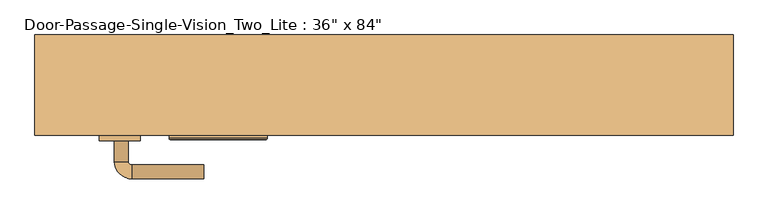
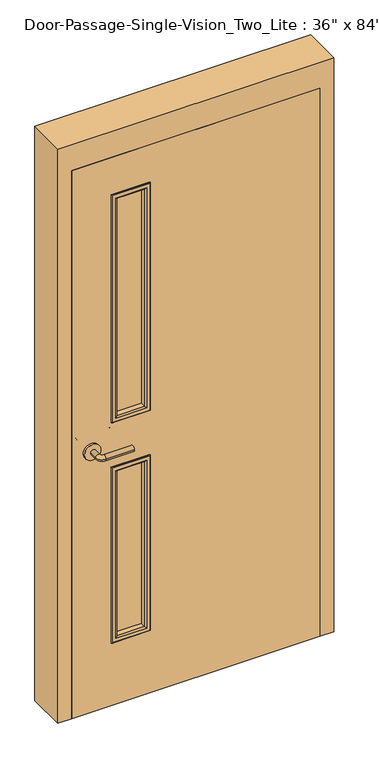
"""IFC4 building model written with IfcOpenShell, lengths in millimetres: door geometry."""

from ifc_helpers import new_model, si_unit, point, frame, frame_2d, origin, place, context, project, spatial, polyline, circle_curve, ellipse_curve, trimmed, segment, composite_curve, outline, extrude, faceted_brep, source, transform, mapped, element, save
from ifc_brep_helpers import plane_surface, cylinder_surface, revolved_surface, advanced_brep


def door_52fb15b9(model_context):
    return source(origin(), model_context, "Body", "SolidModel", [
        advanced_brep(
        [(-392.190625, -68.2, 1016.0), (-372.190625, -68.2, 1016.0), (-392.190625, -38.2, 1016.0), (-372.190625, -38.2, 1016.0), (-367.190625, -33.2, 1016.0), (-367.190625, -13.2, 1016.0), (-262.190625, -13.2, 1016.0), (-262.190625, -33.2, 1016.0)],
        [
            (0, 1, circle_curve(frame((-382.190625, -68.2, 1016.0), z_axis=(0.0, -1.0, 0.0), x_axis=(1.0, 0.0, 0.0)), 10.0)),
            (1, 0, circle_curve(frame((-382.190625, -68.2, 1016.0), z_axis=(0.0, -1.0, 0.0), x_axis=(1.0, 0.0, 0.0)), 10.0)),
            (0, 2),
            (2, 3, circle_curve(frame((-382.190625, -38.2, 1016.0), z_axis=(0.0, -1.0, 0.0), x_axis=(1.0, 0.0, 0.0)), 10.0)),
            (3, 1),
            (3, 2, circle_curve(frame((-382.190625, -38.2, 1016.0), z_axis=(0.0, -1.0, 0.0), x_axis=(1.0, 0.0, 0.0)), 10.0)),
            (4, 3, circle_curve(frame((-367.190625, -38.2, 1016.0), z_axis=(0.0, 0.0, 1.0), x_axis=(-1.0, 0.0, 0.0)), 5.0)),
            (2, 5, circle_curve(frame((-367.190625, -38.2, 1016.0), z_axis=(0.0, 0.0, -1.0), x_axis=(-1.0, 0.0, 0.0)), 25.0)),
            (5, 4, circle_curve(frame((-367.190625, -23.2, 1016.0), z_axis=(-1.0, 0.0, 0.0), x_axis=(0.0, -1.0, 0.0)), 10.0)),
            (4, 5, circle_curve(frame((-367.190625, -23.2, 1016.0), z_axis=(-1.0, 0.0, 0.0), x_axis=(0.0, -1.0, 0.0)), 10.0)),
            (6, 7, circle_curve(frame((-262.190625, -23.2, 1016.0), z_axis=(1.0, 0.0, 0.0), x_axis=(0.0, -1.0, 0.0)), 10.0)),
            (7, 6, circle_curve(frame((-262.190625, -23.2, 1016.0), z_axis=(1.0, 0.0, 0.0), x_axis=(0.0, -1.0, 0.0)), 10.0)),
            (5, 6),
            (7, 4),
        ],
        [
            plane_surface(frame((-382.190625, -68.2, 1016.0), z_axis=(0.0, -1.0, 0.0), x_axis=(0.0, 0.0, 1.0))),
            cylinder_surface(frame((-382.190625, -68.2, 1016.0), z_axis=(0.0, -1.0, 0.0), x_axis=(1.0, 0.0, 0.0)), 10.0),
            revolved_surface(trimmed(ellipse_curve(frame((-382.190625, -38.2, 1016.0), z_axis=(0.0, -1.0, 0.0), x_axis=(1.0, 0.0, 0.0)), 10.0, 10.0), [point((-392.190625, -38.2, 1016.0))], [point((-372.190625, -38.2, 1016.0))], True, "CARTESIAN"), (-367.190625, -38.2, 1016.0), (0.0, 0.0, -1.0)),
            revolved_surface(trimmed(ellipse_curve(frame((-382.190625, -38.2, 1016.0), z_axis=(0.0, -1.0, 0.0), x_axis=(1.0, 0.0, 0.0)), 10.0, 10.0), [point((-372.190625, -38.2, 1016.0))], [point((-392.190625, -38.2, 1016.0))], True, "CARTESIAN"), (-367.190625, -38.2, 1016.0), (0.0, 0.0, -1.0)),
            plane_surface(frame((-262.190625, -23.2, 1016.0), z_axis=(1.0, 0.0, 0.0), x_axis=(0.0, 0.0, 1.0))),
            cylinder_surface(frame((-367.190625, -23.2, 1016.0), z_axis=(-1.0, 0.0, 0.0), x_axis=(0.0, -1.0, 0.0)), 10.0),
        ],
        [
            (0, [[1, 2]]),
            (1, [[-1, 3, 4, 5]]),
            (1, [[-2, -5, 6, -3]]),
            (2, [[7, -4, 8, 9]]),
            (3, [[-8, -6, -7, 10]]),
            (4, [[11, 12]]),
            (5, [[-9, 13, -12, 14]]),
            (5, [[-10, -14, -11, -13]]),
        ],
    ),
        extrude(outline(composite_curve([segment(trimmed(circle_curve(frame_2d((1016.0, -384.690625)), 30.0), [point((1016.0, -414.690625))], [point((1016.0, -354.690625))], False, "CARTESIAN"), True, "CONTINUOUS"), segment(trimmed(circle_curve(frame_2d((1016.0, -384.690625)), 30.0), [point((1016.0, -354.690625))], [point((1016.0, -414.690625))], False, "CARTESIAN"), True, "CONTINUOUS")], self_intersect=False)), frame((0.0, -76.2, 0.0), z_axis=(0.0, 1.0, 0.0), x_axis=(0.0, 0.0, 1.0)), (0.0, 0.0, 1.0), 8.0),
        advanced_brep(
        [(-392.190625, -128.65, 1016.0), (-372.190625, -128.65, 1016.0), (-372.190625, -158.65, 1016.0), (-392.190625, -158.65, 1016.0), (-367.190625, -163.65, 1016.0), (-367.190625, -183.65, 1016.0), (-262.190625, -183.65, 1016.0), (-262.190625, -163.65, 1016.0)],
        [
            (0, 1, circle_curve(frame((-382.190625, -128.65, 1016.0), z_axis=(0.0, 1.0, 0.0), x_axis=(1.0, 0.0, 0.0)), 10.0)),
            (1, 0, circle_curve(frame((-382.190625, -128.65, 1016.0), z_axis=(0.0, 1.0, 0.0), x_axis=(1.0, 0.0, 0.0)), 10.0)),
            (1, 2),
            (2, 3, circle_curve(frame((-382.190625, -158.65, 1016.0), z_axis=(0.0, 1.0, 0.0), x_axis=(1.0, 0.0, 0.0)), 10.0)),
            (3, 0),
            (3, 2, circle_curve(frame((-382.190625, -158.65, 1016.0), z_axis=(0.0, 1.0, 0.0), x_axis=(1.0, 0.0, 0.0)), 10.0)),
            (4, 5, circle_curve(frame((-367.190625, -173.65, 1016.0), z_axis=(-1.0, 0.0, 0.0), x_axis=(0.0, 1.0, 0.0)), 10.0)),
            (5, 3, circle_curve(frame((-367.190625, -158.65, 1016.0), z_axis=(0.0, 0.0, -1.0), x_axis=(-1.0, 0.0, 0.0)), 25.0)),
            (2, 4, circle_curve(frame((-367.190625, -158.65, 1016.0), z_axis=(0.0, 0.0, 1.0), x_axis=(-1.0, 0.0, 0.0)), 5.0)),
            (5, 4, circle_curve(frame((-367.190625, -173.65, 1016.0), z_axis=(-1.0, 0.0, 0.0), x_axis=(0.0, 1.0, 0.0)), 10.0)),
            (6, 7, circle_curve(frame((-262.190625, -173.65, 1016.0), z_axis=(1.0, 0.0, 0.0), x_axis=(0.0, 1.0, 0.0)), 10.0)),
            (7, 6, circle_curve(frame((-262.190625, -173.65, 1016.0), z_axis=(1.0, 0.0, 0.0), x_axis=(0.0, 1.0, 0.0)), 10.0)),
            (4, 7),
            (6, 5),
        ],
        [
            plane_surface(frame((-382.190625, -128.65, 1016.0), z_axis=(0.0, 1.0, 0.0), x_axis=(0.0, 0.0, 1.0))),
            cylinder_surface(frame((-382.190625, -128.65, 1016.0), z_axis=(0.0, 1.0, 0.0), x_axis=(1.0, 0.0, 0.0)), 10.0),
            revolved_surface(trimmed(ellipse_curve(frame((-382.190625, -158.65, 1016.0), z_axis=(0.0, -1.0, 0.0), x_axis=(1.0, 0.0, 0.0)), 10.0, 10.0), [point((-392.190625, -158.65, 1016.0))], [point((-372.190625, -158.65, 1016.0))], True, "CARTESIAN"), (-367.190625, -158.65, 1016.0), (0.0, 0.0, -1.0)),
            revolved_surface(trimmed(ellipse_curve(frame((-382.190625, -158.65, 1016.0), z_axis=(0.0, -1.0, 0.0), x_axis=(1.0, 0.0, 0.0)), 10.0, 10.0), [point((-372.190625, -158.65, 1016.0))], [point((-392.190625, -158.65, 1016.0))], True, "CARTESIAN"), (-367.190625, -158.65, 1016.0), (0.0, 0.0, -1.0)),
            plane_surface(frame((-262.190625, -173.65, 1016.0), z_axis=(1.0, 0.0, 0.0), x_axis=(0.0, 0.0, 1.0))),
            cylinder_surface(frame((-367.190625, -173.65, 1016.0), z_axis=(-1.0, 0.0, 0.0), x_axis=(0.0, 1.0, 0.0)), 10.0),
        ],
        [
            (0, [[1, 2]]),
            (1, [[3, 4, 5, -2]]),
            (1, [[-5, 6, -3, -1]]),
            (2, [[7, 8, -4, 9]]),
            (3, [[10, -9, -6, -8]]),
            (4, [[11, 12]]),
            (5, [[13, -11, 14, -7]]),
            (5, [[-14, -12, -13, -10]]),
        ],
    ),
        extrude(outline(composite_curve([segment(trimmed(circle_curve(frame_2d((1016.0, -384.690625)), 30.0), [point((1016.0, -414.690625))], [point((1016.0, -354.690625))], False, "CARTESIAN"), True, "CONTINUOUS"), segment(trimmed(circle_curve(frame_2d((1016.0, -384.690625)), 30.0), [point((1016.0, -354.690625))], [point((1016.0, -414.690625))], False, "CARTESIAN"), True, "CONTINUOUS")], self_intersect=False)), frame((0.0, -128.65, 0.0), z_axis=(0.0, 1.0, 0.0), x_axis=(0.0, 0.0, 1.0)), (0.0, 0.0, 1.0), 8.0),
        extrude(outline(polyline([(2133.6, -457.2), (0.0, -457.2), (0.0, 457.2), (2133.6, 457.2), (2133.6, -457.2)]), holes=[polyline([(1981.2, -304.8), (1981.2, -177.8), (1111.25, -177.8), (1111.25, -304.8), (1981.2, -304.8)]), polyline([(920.75, -304.8), (920.75, -177.8), (254.0, -177.8), (254.0, -304.8), (920.75, -304.8)])]), frame((0.0, -120.65, 0.0), z_axis=(0.0, 1.0, 0.0), x_axis=(0.0, 0.0, 1.0)), (0.0, 0.0, 1.0), 44.45),
        faceted_brep([(457.2, -71.4375, 0.0), (441.325, -71.4375, 0.0), (441.325, -23.8125, 0.0), (457.2, -23.8125, 0.0), (457.2, 25.4, 0.0), (508.0, 25.4, 0.0), (508.0, -120.65, 0.0), (457.2, -120.65, 0.0), (457.2, -120.65, 2133.6), (457.2, -71.4375, 2133.6), (508.0, -120.65, 2235.2), (-508.0, -120.65, 2235.2), (-508.0, -120.65, 0.0), (-457.2, -120.65, 0.0), (-457.2, -120.65, 2133.6), (508.0, 25.4, 2235.2), (457.2, 25.4, 2133.6), (-457.2, 25.4, 2133.6), (-457.2, 25.4, 0.0), (-508.0, 25.4, 0.0), (-508.0, 25.4, 2235.2), (457.2, -23.8125, 2133.6), (441.325, -23.8125, 2117.725), (-441.325, -23.8125, 2117.725), (-441.325, -23.8125, 0.0), (-457.2, -23.8125, 0.0), (-457.2, -23.8125, 2133.6), (441.325, -71.4375, 2117.725), (-457.2, -71.4375, 2133.6), (-457.2, -71.4375, 0.0), (-441.325, -71.4375, 0.0), (-441.325, -71.4375, 2117.725)], [[[0, 1, 2, 3, 4, 5, 6, 7]], [[7, 8, 9, 0]], [[6, 10, 11, 12, 13, 14, 8, 7]], [[5, 15, 10, 6]], [[4, 16, 17, 18, 19, 20, 15, 5]], [[3, 21, 16, 4]], [[2, 22, 23, 24, 25, 26, 21, 3]], [[1, 27, 22, 2]], [[0, 9, 28, 29, 30, 31, 27, 1]], [[8, 14, 28, 9]], [[16, 21, 26, 17]], [[22, 27, 31, 23]], [[12, 19, 18, 25, 24, 30, 29, 13]], [[13, 29, 28, 14]], [[11, 20, 19, 12]], [[17, 26, 25, 18]], [[23, 31, 30, 24]], [[15, 20, 11, 10]]]),
        extrude(outline(polyline([(-177.8, -95.25), (-177.8, -101.6), (-304.8, -101.6), (-304.8, -95.25), (-177.8, -95.25)])), frame((0.0, 0.0, 1111.25), z_axis=(0.0, 0.0, 1.0), x_axis=(1.0, 0.0, 0.0)), (0.0, 0.0, 1.0), 869.95),
        extrude(outline(polyline([(-177.8, -95.25), (-177.8, -101.6), (-304.8, -101.6), (-304.8, -95.25), (-177.8, -95.25)])), frame((0.0, 0.0, 254.0), z_axis=(0.0, 0.0, 1.0), x_axis=(1.0, 0.0, 0.0)), (0.0, 0.0, 1.0), 666.75),
        advanced_brep(
        [(-304.8, -101.6, 1981.2), (-304.8, -101.6, 1111.25), (-304.8, -120.65, 1111.25), (-304.8, -120.65, 1981.2), (-292.8, -121.65, 1969.2), (-292.8, -121.65, 1123.25), (-292.8, -101.6, 1123.25), (-292.8, -101.6, 1969.2), (-297.8, -126.65, 1974.2), (-297.8, -126.65, 1118.25), (-312.8, -124.65, 1989.2), (-312.8, -124.65, 1103.25), (-310.8, -126.65, 1105.25), (-310.8, -126.65, 1987.2), (-312.8, -120.65, 1989.2), (-312.8, -120.65, 1103.25), (-177.8, -101.6, 1111.25), (-177.8, -120.65, 1111.25), (-189.8, -121.65, 1123.25), (-189.8, -101.6, 1123.25), (-184.8, -126.65, 1118.25), (-169.8, -124.65, 1103.25), (-171.8, -126.65, 1105.25), (-169.8, -120.65, 1103.25), (-177.8, -101.6, 1981.2), (-177.8, -120.65, 1981.2), (-189.8, -121.65, 1969.2), (-189.8, -101.6, 1969.2), (-184.8, -126.65, 1974.2), (-169.8, -124.65, 1989.2), (-171.8, -126.65, 1987.2), (-169.8, -120.65, 1989.2)],
        [
            (0, 1),
            (1, 2),
            (2, 3),
            (3, 0),
            (4, 5),
            (5, 6),
            (6, 7),
            (7, 4),
            (8, 9),
            (9, 5, ellipse_curve(frame((-297.8, -121.65, 1118.25), z_axis=(-0.7071067811865475, 0.0, 0.7071067811865475), x_axis=(0.7071067811865474, 0.0, 0.7071067811865476)), 7.0710678, 5.0)),
            (4, 8, ellipse_curve(frame((-297.8, -121.65, 1974.2), z_axis=(-0.7071067811865475, 0.0, -0.7071067811865475), x_axis=(-0.7071067811865474, 0.0, 0.7071067811865476)), 7.0710678, 5.0)),
            (10, 11),
            (11, 12, ellipse_curve(frame((-310.8, -124.65, 1105.25), z_axis=(-0.7071067811865475, 0.0, 0.7071067811865475), x_axis=(0.7071067811865474, 0.0, 0.7071067811865476)), 2.8284271, 2.0)),
            (12, 13),
            (13, 10, ellipse_curve(frame((-310.8, -124.65, 1987.2), z_axis=(-0.7071067811865475, 0.0, -0.7071067811865475), x_axis=(-0.7071067811865474, 0.0, 0.7071067811865476)), 2.8284271, 2.0)),
            (14, 15),
            (15, 11),
            (10, 14),
            (1, 16),
            (16, 17),
            (17, 2),
            (5, 18),
            (18, 19),
            (19, 6),
            (9, 20),
            (20, 18, ellipse_curve(frame((-184.8, -121.65, 1118.25), z_axis=(-0.7071067811865475, 0.0, -0.7071067811865475), x_axis=(-0.7071067811865476, 0.0, 0.7071067811865474)), 7.0710678, 5.0)),
            (11, 21),
            (21, 22, ellipse_curve(frame((-171.8, -124.65, 1105.25), z_axis=(-0.7071067811865475, 0.0, -0.7071067811865475), x_axis=(-0.7071067811865476, 0.0, 0.7071067811865474)), 2.8284271, 2.0)),
            (22, 12),
            (15, 23),
            (23, 21),
            (16, 24),
            (24, 25),
            (25, 17),
            (18, 26),
            (26, 27),
            (27, 19),
            (20, 28),
            (28, 26, ellipse_curve(frame((-184.8, -121.65, 1974.2), z_axis=(0.7071067811865475, 0.0, -0.7071067811865475), x_axis=(-0.7071067811865474, 0.0, -0.7071067811865476)), 7.0710678, 5.0)),
            (21, 29),
            (29, 30, ellipse_curve(frame((-171.8, -124.65, 1987.2), z_axis=(0.7071067811865475, 0.0, -0.7071067811865475), x_axis=(-0.7071067811865474, 0.0, -0.7071067811865476)), 2.8284271, 2.0)),
            (30, 22),
            (23, 31),
            (31, 29),
            (14, 31),
            (25, 3),
            (24, 0),
            (27, 7),
            (26, 4),
            (28, 8),
            (30, 13),
            (29, 10),
        ],
        [
            plane_surface(frame((-304.8, -120.65, 1981.2), z_axis=(-1.0, 0.0, 0.0), x_axis=(0.0, 0.0, -1.0))),
            plane_surface(frame((-292.8, -101.6, 1969.2), z_axis=(1.0, 0.0, 0.0), x_axis=(0.0, 0.0, -1.0))),
            cylinder_surface(frame((-297.8, -121.65, 1981.2), z_axis=(0.0, 0.0, 1.0), x_axis=(-1.0, 0.0, 0.0)), 5.0),
            cylinder_surface(frame((-310.8, -124.65, 1981.2), z_axis=(0.0, 0.0, 1.0), x_axis=(-1.0, 0.0, 0.0)), 2.0),
            plane_surface(frame((-312.8, -124.65, 1989.2), z_axis=(-1.0, 0.0, 0.0), x_axis=(0.0, 0.0, -1.0))),
            plane_surface(frame((-304.8, -120.65, 1111.25), z_axis=(0.0, 0.0, -1.0), x_axis=(1.0, 0.0, 0.0))),
            plane_surface(frame((-292.8, -101.6, 1123.25), z_axis=(0.0, 0.0, 1.0), x_axis=(1.0, 0.0, 0.0))),
            cylinder_surface(frame((-304.8, -121.65, 1118.25), z_axis=(-1.0, 0.0, 0.0), x_axis=(0.0, 0.0, -1.0)), 5.0),
            cylinder_surface(frame((-304.8, -124.65, 1105.25), z_axis=(-1.0, 0.0, 0.0), x_axis=(0.0, 0.0, -1.0)), 2.0),
            plane_surface(frame((-312.8, -124.65, 1103.25), z_axis=(0.0, 0.0, -1.0), x_axis=(1.0, 0.0, 0.0))),
            plane_surface(frame((-177.8, -120.65, 1111.25), z_axis=(1.0, 0.0, 0.0), x_axis=(0.0, 0.0, 1.0))),
            plane_surface(frame((-189.8, -101.6, 1123.25), z_axis=(-1.0, 0.0, 0.0), x_axis=(0.0, 0.0, 1.0))),
            cylinder_surface(frame((-184.8, -121.65, 1111.25), z_axis=(0.0, 0.0, -1.0), x_axis=(1.0, 0.0, 0.0)), 5.0),
            cylinder_surface(frame((-171.8, -124.65, 1111.25), z_axis=(0.0, 0.0, -1.0), x_axis=(1.0, 0.0, 0.0)), 2.0),
            plane_surface(frame((-169.8, -124.65, 1103.25), z_axis=(1.0, 0.0, 0.0), x_axis=(0.0, 0.0, 1.0))),
            plane_surface(frame((-169.8, -120.65, 1989.2), z_axis=(0.0, 1.0, 0.0), x_axis=(-1.0, 0.0, 0.0))),
            plane_surface(frame((-177.8, -120.65, 1981.2), z_axis=(0.0, 0.0, 1.0), x_axis=(-1.0, 0.0, 0.0))),
            plane_surface(frame((-177.8, -101.6, 1981.2), z_axis=(0.0, 1.0, 0.0), x_axis=(-1.0, 0.0, 0.0))),
            plane_surface(frame((-189.8, -101.6, 1969.2), z_axis=(0.0, 0.0, -1.0), x_axis=(-1.0, 0.0, 0.0))),
            cylinder_surface(frame((-177.8, -121.65, 1974.2), z_axis=(1.0, 0.0, 0.0), x_axis=(0.0, 0.0, 1.0)), 5.0),
            plane_surface(frame((-184.8, -126.65, 1974.2), z_axis=(0.0, -1.0, 0.0), x_axis=(-1.0, 0.0, 0.0))),
            cylinder_surface(frame((-177.8, -124.65, 1987.2), z_axis=(1.0, 0.0, 0.0), x_axis=(0.0, 0.0, 1.0)), 2.0),
            plane_surface(frame((-169.8, -124.65, 1989.2), z_axis=(0.0, 0.0, 1.0), x_axis=(-1.0, 0.0, 0.0))),
        ],
        [
            (0, [[1, 2, 3, 4]]),
            (1, [[5, 6, 7, 8]]),
            (2, [[9, 10, -5, 11]]),
            (3, [[12, 13, 14, 15]]),
            (4, [[16, 17, -12, 18]]),
            (5, [[19, 20, 21, -2]]),
            (6, [[22, 23, 24, -6]]),
            (7, [[25, 26, -22, -10]]),
            (8, [[27, 28, 29, -13]]),
            (9, [[30, 31, -27, -17]]),
            (10, [[32, 33, 34, -20]]),
            (11, [[35, 36, 37, -23]]),
            (12, [[38, 39, -35, -26]]),
            (13, [[40, 41, 42, -28]]),
            (14, [[43, 44, -40, -31]]),
            (15, [[-16, 45, -43, -30], [-3, -21, -34, 46]]),
            (16, [[47, -4, -46, -33]]),
            (17, [[-1, -47, -32, -19], [-7, -24, -37, 48]]),
            (18, [[49, -8, -48, -36]]),
            (19, [[50, -11, -49, -39]]),
            (20, [[-14, -29, -42, 51], [-9, -50, -38, -25]]),
            (21, [[52, -15, -51, -41]]),
            (22, [[-45, -18, -52, -44]]),
        ],
    ),
        advanced_brep(
        [(-304.8, -95.25, 1111.25), (-304.8, -95.25, 1981.2), (-304.8, -76.2, 1981.2), (-304.8, -76.2, 1111.25), (-292.8, -75.2, 1123.25), (-292.8, -75.2, 1969.2), (-292.8, -95.25, 1969.2), (-292.8, -95.25, 1123.25), (-297.8, -70.2, 1118.25), (-297.8, -70.2, 1974.2), (-312.8, -72.2, 1103.25), (-312.8, -72.2, 1989.2), (-310.8, -70.2, 1987.2), (-310.8, -70.2, 1105.25), (-312.8, -76.2, 1103.25), (-312.8, -76.2, 1989.2), (-177.8, -95.25, 1981.2), (-177.8, -76.2, 1981.2), (-189.8, -75.2, 1969.2), (-189.8, -95.25, 1969.2), (-184.8, -70.2, 1974.2), (-169.8, -72.2, 1989.2), (-171.8, -70.2, 1987.2), (-169.8, -76.2, 1989.2), (-177.8, -95.25, 1111.25), (-177.8, -76.2, 1111.25), (-189.8, -75.2, 1123.25), (-189.8, -95.25, 1123.25), (-184.8, -70.2, 1118.25), (-169.8, -72.2, 1103.25), (-171.8, -70.2, 1105.25), (-169.8, -76.2, 1103.25)],
        [
            (0, 1),
            (1, 2),
            (2, 3),
            (3, 0),
            (4, 5),
            (5, 6),
            (6, 7),
            (7, 4),
            (8, 9),
            (9, 5, ellipse_curve(frame((-297.8, -75.2, 1974.2), z_axis=(-0.7071067811865475, 0.0, -0.7071067811865475), x_axis=(0.7071067811865474, 0.0, -0.7071067811865476)), 7.0710678, 5.0)),
            (4, 8, ellipse_curve(frame((-297.8, -75.2, 1118.25), z_axis=(-0.7071067811865475, 0.0, 0.7071067811865475), x_axis=(-0.7071067811865474, 0.0, -0.7071067811865476)), 7.0710678, 5.0)),
            (10, 11),
            (11, 12, ellipse_curve(frame((-310.8, -72.2, 1987.2), z_axis=(-0.7071067811865475, 0.0, -0.7071067811865475), x_axis=(0.7071067811865474, 0.0, -0.7071067811865476)), 2.8284271, 2.0)),
            (12, 13),
            (13, 10, ellipse_curve(frame((-310.8, -72.2, 1105.25), z_axis=(-0.7071067811865475, 0.0, 0.7071067811865475), x_axis=(-0.7071067811865474, 0.0, -0.7071067811865476)), 2.8284271, 2.0)),
            (14, 15),
            (15, 11),
            (10, 14),
            (1, 16),
            (16, 17),
            (17, 2),
            (5, 18),
            (18, 19),
            (19, 6),
            (9, 20),
            (20, 18, ellipse_curve(frame((-184.8, -75.2, 1974.2), z_axis=(-0.7071067811865475, 0.0, 0.7071067811865475), x_axis=(-0.7071067811865476, 0.0, -0.7071067811865474)), 7.0710678, 5.0)),
            (11, 21),
            (21, 22, ellipse_curve(frame((-171.8, -72.2, 1987.2), z_axis=(-0.7071067811865475, 0.0, 0.7071067811865475), x_axis=(-0.7071067811865476, 0.0, -0.7071067811865474)), 2.8284271, 2.0)),
            (22, 12),
            (15, 23),
            (23, 21),
            (16, 24),
            (24, 25),
            (25, 17),
            (18, 26),
            (26, 27),
            (27, 19),
            (20, 28),
            (28, 26, ellipse_curve(frame((-184.8, -75.2, 1118.25), z_axis=(0.7071067811865475, 0.0, 0.7071067811865475), x_axis=(-0.7071067811865474, 0.0, 0.7071067811865476)), 7.0710678, 5.0)),
            (21, 29),
            (29, 30, ellipse_curve(frame((-171.8, -72.2, 1105.25), z_axis=(0.7071067811865475, 0.0, 0.7071067811865475), x_axis=(-0.7071067811865474, 0.0, 0.7071067811865476)), 2.8284271, 2.0)),
            (30, 22),
            (23, 31),
            (31, 29),
            (14, 31),
            (25, 3),
            (24, 0),
            (27, 7),
            (26, 4),
            (28, 8),
            (30, 13),
            (29, 10),
        ],
        [
            plane_surface(frame((-304.8, -76.2, 1111.25), z_axis=(-1.0, 0.0, 0.0), x_axis=(0.0, 0.0, 1.0))),
            plane_surface(frame((-292.8, -95.25, 1123.25), z_axis=(1.0, 0.0, 0.0), x_axis=(0.0, 0.0, 1.0))),
            cylinder_surface(frame((-297.8, -75.2, 1111.25), z_axis=(0.0, 0.0, -1.0), x_axis=(-1.0, 0.0, 0.0)), 5.0),
            cylinder_surface(frame((-310.8, -72.2, 1111.25), z_axis=(0.0, 0.0, -1.0), x_axis=(-1.0, 0.0, 0.0)), 2.0),
            plane_surface(frame((-312.8, -72.2, 1103.25), z_axis=(-1.0, 0.0, 0.0), x_axis=(0.0, 0.0, 1.0))),
            plane_surface(frame((-304.8, -76.2, 1981.2), z_axis=(0.0, 0.0, 1.0), x_axis=(1.0, 0.0, 0.0))),
            plane_surface(frame((-292.8, -95.25, 1969.2), z_axis=(0.0, 0.0, -1.0), x_axis=(1.0, 0.0, 0.0))),
            cylinder_surface(frame((-304.8, -75.2, 1974.2), z_axis=(-1.0, 0.0, 0.0), x_axis=(0.0, 0.0, 1.0)), 5.0),
            cylinder_surface(frame((-304.8, -72.2, 1987.2), z_axis=(-1.0, 0.0, 0.0), x_axis=(0.0, 0.0, 1.0)), 2.0),
            plane_surface(frame((-312.8, -72.2, 1989.2), z_axis=(0.0, 0.0, 1.0), x_axis=(1.0, 0.0, 0.0))),
            plane_surface(frame((-177.8, -76.2, 1981.2), z_axis=(1.0, 0.0, 0.0), x_axis=(0.0, 0.0, -1.0))),
            plane_surface(frame((-189.8, -95.25, 1969.2), z_axis=(-1.0, 0.0, 0.0), x_axis=(0.0, 0.0, -1.0))),
            cylinder_surface(frame((-184.8, -75.2, 1981.2), z_axis=(0.0, 0.0, 1.0), x_axis=(1.0, 0.0, 0.0)), 5.0),
            cylinder_surface(frame((-171.8, -72.2, 1981.2), z_axis=(0.0, 0.0, 1.0), x_axis=(1.0, 0.0, 0.0)), 2.0),
            plane_surface(frame((-169.8, -72.2, 1989.2), z_axis=(1.0, 0.0, 0.0), x_axis=(0.0, 0.0, -1.0))),
            plane_surface(frame((-169.8, -76.2, 1103.25), z_axis=(0.0, -1.0, 0.0), x_axis=(-1.0, 0.0, 0.0))),
            plane_surface(frame((-177.8, -76.2, 1111.25), z_axis=(0.0, 0.0, -1.0), x_axis=(-1.0, 0.0, 0.0))),
            plane_surface(frame((-177.8, -95.25, 1111.25), z_axis=(0.0, -1.0, 0.0), x_axis=(-1.0, 0.0, 0.0))),
            plane_surface(frame((-189.8, -95.25, 1123.25), z_axis=(0.0, 0.0, 1.0), x_axis=(-1.0, 0.0, 0.0))),
            cylinder_surface(frame((-177.8, -75.2, 1118.25), z_axis=(1.0, 0.0, 0.0), x_axis=(0.0, 0.0, -1.0)), 5.0),
            plane_surface(frame((-184.8, -70.2, 1118.25), z_axis=(0.0, 1.0, 0.0), x_axis=(-1.0, 0.0, 0.0))),
            cylinder_surface(frame((-177.8, -72.2, 1105.25), z_axis=(1.0, 0.0, 0.0), x_axis=(0.0, 0.0, -1.0)), 2.0),
            plane_surface(frame((-169.8, -72.2, 1103.25), z_axis=(0.0, 0.0, -1.0), x_axis=(-1.0, 0.0, 0.0))),
        ],
        [
            (0, [[1, 2, 3, 4]]),
            (1, [[5, 6, 7, 8]]),
            (2, [[9, 10, -5, 11]]),
            (3, [[12, 13, 14, 15]]),
            (4, [[16, 17, -12, 18]]),
            (5, [[19, 20, 21, -2]]),
            (6, [[22, 23, 24, -6]]),
            (7, [[25, 26, -22, -10]]),
            (8, [[27, 28, 29, -13]]),
            (9, [[30, 31, -27, -17]]),
            (10, [[32, 33, 34, -20]]),
            (11, [[35, 36, 37, -23]]),
            (12, [[38, 39, -35, -26]]),
            (13, [[40, 41, 42, -28]]),
            (14, [[43, 44, -40, -31]]),
            (15, [[-16, 45, -43, -30], [-3, -21, -34, 46]]),
            (16, [[47, -4, -46, -33]]),
            (17, [[-1, -47, -32, -19], [-7, -24, -37, 48]]),
            (18, [[49, -8, -48, -36]]),
            (19, [[50, -11, -49, -39]]),
            (20, [[-14, -29, -42, 51], [-9, -50, -38, -25]]),
            (21, [[52, -15, -51, -41]]),
            (22, [[-45, -18, -52, -44]]),
        ],
    ),
        advanced_brep(
        [(-304.8, -101.6, 920.75), (-304.8, -101.6, 254.0), (-304.8, -120.65, 254.0), (-304.8, -120.65, 920.75), (-292.8, -121.65, 908.75), (-292.8, -121.65, 266.0), (-292.8, -101.6, 266.0), (-292.8, -101.6, 908.75), (-297.8, -126.65, 913.75), (-297.8, -126.65, 261.0), (-312.8, -124.65, 928.75), (-312.8, -124.65, 246.0), (-310.8, -126.65, 248.0), (-310.8, -126.65, 926.75), (-312.8, -120.65, 928.75), (-312.8, -120.65, 246.0), (-177.8, -101.6, 254.0), (-177.8, -120.65, 254.0), (-189.8, -121.65, 266.0), (-189.8, -101.6, 266.0), (-184.8, -126.65, 261.0), (-169.8, -124.65, 246.0), (-171.8, -126.65, 248.0), (-169.8, -120.65, 246.0), (-177.8, -101.6, 920.75), (-177.8, -120.65, 920.75), (-189.8, -121.65, 908.75), (-189.8, -101.6, 908.75), (-184.8, -126.65, 913.75), (-169.8, -124.65, 928.75), (-171.8, -126.65, 926.75), (-169.8, -120.65, 928.75)],
        [
            (0, 1),
            (1, 2),
            (2, 3),
            (3, 0),
            (4, 5),
            (5, 6),
            (6, 7),
            (7, 4),
            (8, 9),
            (9, 5, ellipse_curve(frame((-297.8, -121.65, 261.0), z_axis=(-0.7071067811865475, 0.0, 0.7071067811865475), x_axis=(0.7071067811865474, 0.0, 0.7071067811865476)), 7.0710678, 5.0)),
            (4, 8, ellipse_curve(frame((-297.8, -121.65, 913.75), z_axis=(-0.7071067811865475, 0.0, -0.7071067811865475), x_axis=(-0.7071067811865474, 0.0, 0.7071067811865476)), 7.0710678, 5.0)),
            (10, 11),
            (11, 12, ellipse_curve(frame((-310.8, -124.65, 248.0), z_axis=(-0.7071067811865475, 0.0, 0.7071067811865475), x_axis=(0.7071067811865474, 0.0, 0.7071067811865476)), 2.8284271, 2.0)),
            (12, 13),
            (13, 10, ellipse_curve(frame((-310.8, -124.65, 926.75), z_axis=(-0.7071067811865475, 0.0, -0.7071067811865475), x_axis=(-0.7071067811865474, 0.0, 0.7071067811865476)), 2.8284271, 2.0)),
            (14, 15),
            (15, 11),
            (10, 14),
            (1, 16),
            (16, 17),
            (17, 2),
            (5, 18),
            (18, 19),
            (19, 6),
            (9, 20),
            (20, 18, ellipse_curve(frame((-184.8, -121.65, 261.0), z_axis=(-0.7071067811865475, 0.0, -0.7071067811865475), x_axis=(-0.7071067811865476, 0.0, 0.7071067811865474)), 7.0710678, 5.0)),
            (11, 21),
            (21, 22, ellipse_curve(frame((-171.8, -124.65, 248.0), z_axis=(-0.7071067811865475, 0.0, -0.7071067811865475), x_axis=(-0.7071067811865476, 0.0, 0.7071067811865474)), 2.8284271, 2.0)),
            (22, 12),
            (15, 23),
            (23, 21),
            (16, 24),
            (24, 25),
            (25, 17),
            (18, 26),
            (26, 27),
            (27, 19),
            (20, 28),
            (28, 26, ellipse_curve(frame((-184.8, -121.65, 913.75), z_axis=(0.7071067811865475, 0.0, -0.7071067811865475), x_axis=(-0.7071067811865474, 0.0, -0.7071067811865476)), 7.0710678, 5.0)),
            (21, 29),
            (29, 30, ellipse_curve(frame((-171.8, -124.65, 926.75), z_axis=(0.7071067811865475, 0.0, -0.7071067811865475), x_axis=(-0.7071067811865474, 0.0, -0.7071067811865476)), 2.8284271, 2.0)),
            (30, 22),
            (23, 31),
            (31, 29),
            (14, 31),
            (25, 3),
            (24, 0),
            (27, 7),
            (26, 4),
            (28, 8),
            (30, 13),
            (29, 10),
        ],
        [
            plane_surface(frame((-304.8, -120.65, 920.75), z_axis=(-1.0, 0.0, 0.0), x_axis=(0.0, 0.0, -1.0))),
            plane_surface(frame((-292.8, -101.6, 908.75), z_axis=(1.0, 0.0, 0.0), x_axis=(0.0, 0.0, -1.0))),
            cylinder_surface(frame((-297.8, -121.65, 920.75), z_axis=(0.0, 0.0, 1.0), x_axis=(-1.0, 0.0, 0.0)), 5.0),
            cylinder_surface(frame((-310.8, -124.65, 920.75), z_axis=(0.0, 0.0, 1.0), x_axis=(-1.0, 0.0, 0.0)), 2.0),
            plane_surface(frame((-312.8, -124.65, 928.75), z_axis=(-1.0, 0.0, 0.0), x_axis=(0.0, 0.0, -1.0))),
            plane_surface(frame((-304.8, -120.65, 254.0), z_axis=(0.0, 0.0, -1.0), x_axis=(1.0, 0.0, 0.0))),
            plane_surface(frame((-292.8, -101.6, 266.0), z_axis=(0.0, 0.0, 1.0), x_axis=(1.0, 0.0, 0.0))),
            cylinder_surface(frame((-304.8, -121.65, 261.0), z_axis=(-1.0, 0.0, 0.0), x_axis=(0.0, 0.0, -1.0)), 5.0),
            cylinder_surface(frame((-304.8, -124.65, 248.0), z_axis=(-1.0, 0.0, 0.0), x_axis=(0.0, 0.0, -1.0)), 2.0),
            plane_surface(frame((-312.8, -124.65, 246.0), z_axis=(0.0, 0.0, -1.0), x_axis=(1.0, 0.0, 0.0))),
            plane_surface(frame((-177.8, -120.65, 254.0), z_axis=(1.0, 0.0, 0.0), x_axis=(0.0, 0.0, 1.0))),
            plane_surface(frame((-189.8, -101.6, 266.0), z_axis=(-1.0, 0.0, 0.0), x_axis=(0.0, 0.0, 1.0))),
            cylinder_surface(frame((-184.8, -121.65, 254.0), z_axis=(0.0, 0.0, -1.0), x_axis=(1.0, 0.0, 0.0)), 5.0),
            cylinder_surface(frame((-171.8, -124.65, 254.0), z_axis=(0.0, 0.0, -1.0), x_axis=(1.0, 0.0, 0.0)), 2.0),
            plane_surface(frame((-169.8, -124.65, 246.0), z_axis=(1.0, 0.0, 0.0), x_axis=(0.0, 0.0, 1.0))),
            plane_surface(frame((-169.8, -120.65, 928.75), z_axis=(0.0, 1.0, 0.0), x_axis=(-1.0, 0.0, 0.0))),
            plane_surface(frame((-177.8, -120.65, 920.75), z_axis=(0.0, 0.0, 1.0), x_axis=(-1.0, 0.0, 0.0))),
            plane_surface(frame((-177.8, -101.6, 920.75), z_axis=(0.0, 1.0, 0.0), x_axis=(-1.0, 0.0, 0.0))),
            plane_surface(frame((-189.8, -101.6, 908.75), z_axis=(0.0, 0.0, -1.0), x_axis=(-1.0, 0.0, 0.0))),
            cylinder_surface(frame((-177.8, -121.65, 913.75), z_axis=(1.0, 0.0, 0.0), x_axis=(0.0, 0.0, 1.0)), 5.0),
            plane_surface(frame((-184.8, -126.65, 913.75), z_axis=(0.0, -1.0, 0.0), x_axis=(-1.0, 0.0, 0.0))),
            cylinder_surface(frame((-177.8, -124.65, 926.75), z_axis=(1.0, 0.0, 0.0), x_axis=(0.0, 0.0, 1.0)), 2.0),
            plane_surface(frame((-169.8, -124.65, 928.75), z_axis=(0.0, 0.0, 1.0), x_axis=(-1.0, 0.0, 0.0))),
        ],
        [
            (0, [[1, 2, 3, 4]]),
            (1, [[5, 6, 7, 8]]),
            (2, [[9, 10, -5, 11]]),
            (3, [[12, 13, 14, 15]]),
            (4, [[16, 17, -12, 18]]),
            (5, [[19, 20, 21, -2]]),
            (6, [[22, 23, 24, -6]]),
            (7, [[25, 26, -22, -10]]),
            (8, [[27, 28, 29, -13]]),
            (9, [[30, 31, -27, -17]]),
            (10, [[32, 33, 34, -20]]),
            (11, [[35, 36, 37, -23]]),
            (12, [[38, 39, -35, -26]]),
            (13, [[40, 41, 42, -28]]),
            (14, [[43, 44, -40, -31]]),
            (15, [[-16, 45, -43, -30], [-3, -21, -34, 46]]),
            (16, [[47, -4, -46, -33]]),
            (17, [[-1, -47, -32, -19], [-7, -24, -37, 48]]),
            (18, [[49, -8, -48, -36]]),
            (19, [[50, -11, -49, -39]]),
            (20, [[-14, -29, -42, 51], [-9, -50, -38, -25]]),
            (21, [[52, -15, -51, -41]]),
            (22, [[-45, -18, -52, -44]]),
        ],
    ),
        advanced_brep(
        [(-177.8, -95.25, 920.75), (-177.8, -95.25, 254.0), (-177.8, -76.2, 254.0), (-177.8, -76.2, 920.75), (-189.8, -75.2, 908.75), (-189.8, -75.2, 266.0), (-189.8, -95.25, 266.0), (-189.8, -95.25, 908.75), (-184.8, -70.2, 913.75), (-184.8, -70.2, 261.0), (-169.8, -72.2, 928.75), (-169.8, -72.2, 246.0), (-171.8, -70.2, 248.0), (-171.8, -70.2, 926.75), (-169.8, -76.2, 928.75), (-169.8, -76.2, 246.0), (-304.8, -95.25, 254.0), (-304.8, -76.2, 254.0), (-292.8, -75.2, 266.0), (-292.8, -95.25, 266.0), (-297.8, -70.2, 261.0), (-312.8, -72.2, 246.0), (-310.8, -70.2, 248.0), (-312.8, -76.2, 246.0), (-304.8, -95.25, 920.75), (-304.8, -76.2, 920.75), (-292.8, -75.2, 908.75), (-292.8, -95.25, 908.75), (-297.8, -70.2, 913.75), (-312.8, -72.2, 928.75), (-310.8, -70.2, 926.75), (-312.8, -76.2, 928.75)],
        [
            (0, 1),
            (1, 2),
            (2, 3),
            (3, 0),
            (4, 5),
            (5, 6),
            (6, 7),
            (7, 4),
            (8, 9),
            (9, 5, ellipse_curve(frame((-184.8, -75.2, 261.0), z_axis=(0.7071067811865475, 0.0, 0.7071067811865475), x_axis=(-0.7071067811865474, 0.0, 0.7071067811865476)), 7.0710678, 5.0)),
            (4, 8, ellipse_curve(frame((-184.8, -75.2, 913.75), z_axis=(0.7071067811865475, 0.0, -0.7071067811865475), x_axis=(0.7071067811865474, 0.0, 0.7071067811865476)), 7.0710678, 5.0)),
            (10, 11),
            (11, 12, ellipse_curve(frame((-171.8, -72.2, 248.0), z_axis=(0.7071067811865475, 0.0, 0.7071067811865475), x_axis=(-0.7071067811865474, 0.0, 0.7071067811865476)), 2.8284271, 2.0)),
            (12, 13),
            (13, 10, ellipse_curve(frame((-171.8, -72.2, 926.75), z_axis=(0.7071067811865475, 0.0, -0.7071067811865475), x_axis=(0.7071067811865474, 0.0, 0.7071067811865476)), 2.8284271, 2.0)),
            (14, 15),
            (15, 11),
            (10, 14),
            (1, 16),
            (16, 17),
            (17, 2),
            (5, 18),
            (18, 19),
            (19, 6),
            (9, 20),
            (20, 18, ellipse_curve(frame((-297.8, -75.2, 261.0), z_axis=(0.7071067811865475, 0.0, -0.7071067811865475), x_axis=(0.7071067811865476, 0.0, 0.7071067811865474)), 7.0710678, 5.0)),
            (11, 21),
            (21, 22, ellipse_curve(frame((-310.8, -72.2, 248.0), z_axis=(0.7071067811865475, 0.0, -0.7071067811865475), x_axis=(0.7071067811865476, 0.0, 0.7071067811865474)), 2.8284271, 2.0)),
            (22, 12),
            (15, 23),
            (23, 21),
            (16, 24),
            (24, 25),
            (25, 17),
            (18, 26),
            (26, 27),
            (27, 19),
            (20, 28),
            (28, 26, ellipse_curve(frame((-297.8, -75.2, 913.75), z_axis=(-0.7071067811865475, 0.0, -0.7071067811865475), x_axis=(0.7071067811865474, 0.0, -0.7071067811865476)), 7.0710678, 5.0)),
            (21, 29),
            (29, 30, ellipse_curve(frame((-310.8, -72.2, 926.75), z_axis=(-0.7071067811865475, 0.0, -0.7071067811865475), x_axis=(0.7071067811865474, 0.0, -0.7071067811865476)), 2.8284271, 2.0)),
            (30, 22),
            (23, 31),
            (31, 29),
            (14, 31),
            (25, 3),
            (24, 0),
            (27, 7),
            (26, 4),
            (28, 8),
            (30, 13),
            (29, 10),
        ],
        [
            plane_surface(frame((-177.8, -76.2, 920.75), z_axis=(1.0, 0.0, 0.0), x_axis=(0.0, 0.0, -1.0))),
            plane_surface(frame((-189.8, -95.25, 908.75), z_axis=(-1.0, 0.0, 0.0), x_axis=(0.0, 0.0, -1.0))),
            cylinder_surface(frame((-184.8, -75.2, 920.75), z_axis=(0.0, 0.0, 1.0), x_axis=(1.0, 0.0, 0.0)), 5.0),
            cylinder_surface(frame((-171.8, -72.2, 920.75), z_axis=(0.0, 0.0, 1.0), x_axis=(1.0, 0.0, 0.0)), 2.0),
            plane_surface(frame((-169.8, -72.2, 928.75), z_axis=(1.0, 0.0, 0.0), x_axis=(0.0, 0.0, -1.0))),
            plane_surface(frame((-177.8, -76.2, 254.0), z_axis=(0.0, 0.0, -1.0), x_axis=(-1.0, 0.0, 0.0))),
            plane_surface(frame((-189.8, -95.25, 266.0), z_axis=(0.0, 0.0, 1.0), x_axis=(-1.0, 0.0, 0.0))),
            cylinder_surface(frame((-177.8, -75.2, 261.0), z_axis=(1.0, 0.0, 0.0), x_axis=(0.0, 0.0, -1.0)), 5.0),
            cylinder_surface(frame((-177.8, -72.2, 248.0), z_axis=(1.0, 0.0, 0.0), x_axis=(0.0, 0.0, -1.0)), 2.0),
            plane_surface(frame((-169.8, -72.2, 246.0), z_axis=(0.0, 0.0, -1.0), x_axis=(-1.0, 0.0, 0.0))),
            plane_surface(frame((-304.8, -76.2, 254.0), z_axis=(-1.0, 0.0, 0.0), x_axis=(0.0, 0.0, 1.0))),
            plane_surface(frame((-292.8, -95.25, 266.0), z_axis=(1.0, 0.0, 0.0), x_axis=(0.0, 0.0, 1.0))),
            cylinder_surface(frame((-297.8, -75.2, 254.0), z_axis=(0.0, 0.0, -1.0), x_axis=(-1.0, 0.0, 0.0)), 5.0),
            cylinder_surface(frame((-310.8, -72.2, 254.0), z_axis=(0.0, 0.0, -1.0), x_axis=(-1.0, 0.0, 0.0)), 2.0),
            plane_surface(frame((-312.8, -72.2, 246.0), z_axis=(-1.0, 0.0, 0.0), x_axis=(0.0, 0.0, 1.0))),
            plane_surface(frame((-312.8, -76.2, 928.75), z_axis=(0.0, -1.0, 0.0), x_axis=(1.0, 0.0, 0.0))),
            plane_surface(frame((-304.8, -76.2, 920.75), z_axis=(0.0, 0.0, 1.0), x_axis=(1.0, 0.0, 0.0))),
            plane_surface(frame((-304.8, -95.25, 920.75), z_axis=(0.0, -1.0, 0.0), x_axis=(1.0, 0.0, 0.0))),
            plane_surface(frame((-292.8, -95.25, 908.75), z_axis=(0.0, 0.0, -1.0), x_axis=(1.0, 0.0, 0.0))),
            cylinder_surface(frame((-304.8, -75.2, 913.75), z_axis=(-1.0, 0.0, 0.0), x_axis=(0.0, 0.0, 1.0)), 5.0),
            plane_surface(frame((-297.8, -70.2, 913.75), z_axis=(0.0, 1.0, 0.0), x_axis=(1.0, 0.0, 0.0))),
            cylinder_surface(frame((-304.8, -72.2, 926.75), z_axis=(-1.0, 0.0, 0.0), x_axis=(0.0, 0.0, 1.0)), 2.0),
            plane_surface(frame((-312.8, -72.2, 928.75), z_axis=(0.0, 0.0, 1.0), x_axis=(1.0, 0.0, 0.0))),
        ],
        [
            (0, [[1, 2, 3, 4]]),
            (1, [[5, 6, 7, 8]]),
            (2, [[9, 10, -5, 11]]),
            (3, [[12, 13, 14, 15]]),
            (4, [[16, 17, -12, 18]]),
            (5, [[19, 20, 21, -2]]),
            (6, [[22, 23, 24, -6]]),
            (7, [[25, 26, -22, -10]]),
            (8, [[27, 28, 29, -13]]),
            (9, [[30, 31, -27, -17]]),
            (10, [[32, 33, 34, -20]]),
            (11, [[35, 36, 37, -23]]),
            (12, [[38, 39, -35, -26]]),
            (13, [[40, 41, 42, -28]]),
            (14, [[43, 44, -40, -31]]),
            (15, [[-16, 45, -43, -30], [-3, -21, -34, 46]]),
            (16, [[47, -4, -46, -33]]),
            (17, [[-1, -47, -32, -19], [-7, -24, -37, 48]]),
            (18, [[49, -8, -48, -36]]),
            (19, [[50, -11, -49, -39]]),
            (20, [[-14, -29, -42, 51], [-9, -50, -38, -25]]),
            (21, [[52, -15, -51, -41]]),
            (22, [[-45, -18, -52, -44]]),
        ],
    ),
    ])


if __name__ == "__main__":
    model = new_model("IFC4")
    model_context = context("Model", 3, world=origin())
    ifc_project = project(units=[si_unit("LENGTHUNIT", "METRE", prefix="MILLI")], contexts=[model_context])
    site = spatial("IfcSite", under=ifc_project)
    building = spatial("IfcBuilding", under=site)
    placement = place(None, origin())
    door_shape = door_52fb15b9(model_context)
    element("IfcDoor", 1, ObjectType="Door-Passage-Single-Vision_Two_Lite : 36\" x 84\"", at=placement, inside=building, context=model_context, shape_type="MappedRepresentation", body=[
        mapped(door_shape, transform((0.0, 0.0, 0.0), x_axis=(1.0, 0.0, 0.0), y_axis=(0.0, 1.0, 0.0), z_axis=(0.0, 0.0, 1.0))),
    ])
    save(model, "model.ifc")

# Revit data of these elements
# Type "Door-Passage-Single-Vision_Two_Lite : 36\" x 84\""
#   Type Mark = "9"
#   Assembly Code = "B2030100"
#   Analytic Construction = "Wooden"
#   Thickness = 0' - 1 3/4"
#   Thermal Resistance (R) = 2.5876 (h·ft²·°F)/BTU
#   Swing Angle [instance default] = 90.00°
#   Strike Height = 3' - 4"
#   Rough Width [instance default] = 3' - 4"
#   Rough Height [instance default] = 7' - 4"
#   MF Opening Height [instance default] = 0' - 4"
#   MF Opening Width [instance default] = 0' - 4"
#   Heat Transfer Coefficient (U) = 0.3865 BTU/(h·ft²·°F)
#   Inset Calculate [instance default] = 0' - 4"
#   Masonry Inset [instance default] = 0' - 1"
#   Height = 7' - 0"
#   Width = 3' - 0"
#   Masonry Frame Depth = 0' - 5 3/4"
#   Masonry Frame [instance default] = yes
#   Function = 1
#   Dry Wall Frame [instance default] = no
#   Panel Material = Wood - Birch
#   Glazing = Glass
#   Glass Stop Material = Metal - Paint Finish - Grey
#   Frame Material = Metal - Paint Finish - Grey
#   Door Handle Material = Aluminum
#   Visual Light Transmittance = 0
#   Solar Heat Gain Coefficient = 0
#   Wall Closure = (empty or 0)
# Element 1 (IfcDoor, "Door-Passage-Single-Vision_Two_Lite : 36\" x 84\"")
#   Materials on its faces: "Metal - Paint Finish - Grey", "Aluminum", "Wood - Birch", "Glass"
# Materials
#   "Wood - Birch": class "Wood", colour RGB 166 116 52, transparency 0, Cost = 0
#   "Glass": class "Glass", colour RGB 0 128 192, transparency 0.75, Description = "Soda Lime Glass", Cost = 0
#   "Metal - Paint Finish - Grey": class "Paint", colour RGB 104 104 104, transparency 0, Cost = 0
#   "Aluminum": class "Metal", colour RGB 247 247 247, transparency 0, Description = "Aluminum 6061", Cost = 0
